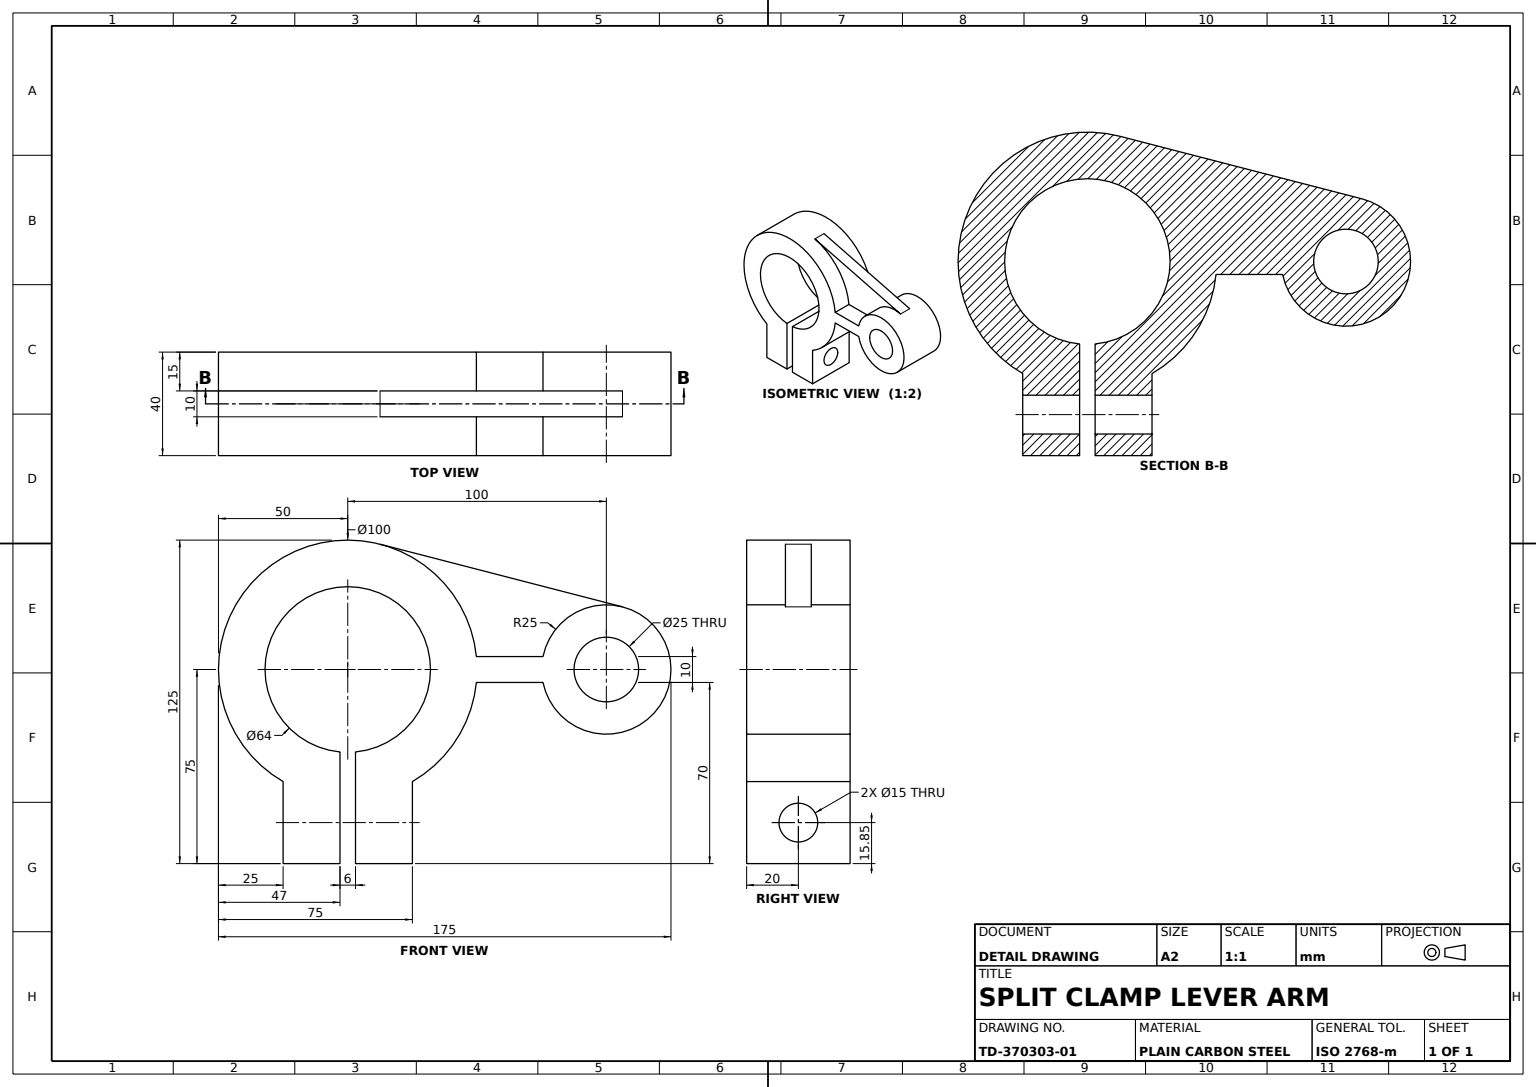
from build123d import *

# Parameters (mm, degrees)
CLAMP_RING_SKETCH_R                       = 50
CLAMP_RING_SKETCH_R_2                     = 32
CLAMP_RING_100_BORE_64_DEPTH              = 20
CLAMP_BLOCK_AND_SECONDARY_BOSS_SKETCH_R   = 25
CLAMP_BLOCK_AND_SECONDARY_BOSS_SKETCH_R_2 = 12.5
CLAMP_BLOCK_AND_SECONDARY_BOSS_SKETCH_W   = 50
CLAMP_BLOCK_AND_SECONDARY_BOSS_SKETCH_H   = 31.698729811
CLAMP_BLOCK_AND_SECONDARY_BOSS_DEPTH      = 20
CLAMP_SLOT_6MM_DEPTH                      = 148.139389696
CLAMP_SLOT_6MM_DEPTH_BACK                 = 148.139389696
CLAMP_SLOT_SKETCH_W                       = 6
CLAMP_SLOT_SKETCH_H                       = 43.140935356
CONNECTING_WEB_SKETCH_W                   = 55.5
CONNECTING_WEB_SKETCH_H                   = 10
CONNECTING_WEB_10MM_DEPTH                 = 20
STIFFENING_RIB_10MM_REACH                 = 149.139
STIFFENING_RIB_SKETCH_WALL_W              = 393.103363046
STIFFENING_RIB_SKETCH_WALL_H              = 10
CLAMP_BOLT_HOLE_15_DEPTH                  = 148.139389696
CLAMP_BOLT_HOLE_15_DEPTH_BACK             = 148.139389696
CLAMP_BOLT_HOLE_SKETCH_R                  = 7.5


with BuildPart() as part:
    # Clamp Ring Sketch → Clamp Ring Ø100 Bore Ø64 (new, symmetric)
    with BuildSketch(Plane.XY):
        Circle(CLAMP_RING_SKETCH_R)
        Circle(CLAMP_RING_SKETCH_R_2, mode=Mode.SUBTRACT)
    extrude(amount=CLAMP_RING_100_BORE_64_DEPTH, both=True)

    # Clamp Block and Secondary Boss Sketch → Clamp Block and Secondary Boss (add, symmetric)
    # profile 1 of 2: a face of its own
    with BuildSketch(Plane.XY):
        with Locations((100, 0)):
            Circle(CLAMP_BLOCK_AND_SECONDARY_BOSS_SKETCH_R)
        with Locations((100, 0)):
            Circle(CLAMP_BLOCK_AND_SECONDARY_BOSS_SKETCH_R_2, mode=Mode.SUBTRACT)
    # profile 2 of 2: a face of its own
    with BuildSketch(Plane.XY):
        with Locations((0, -59.150635095)):
            Rectangle(CLAMP_BLOCK_AND_SECONDARY_BOSS_SKETCH_W, CLAMP_BLOCK_AND_SECONDARY_BOSS_SKETCH_H)
    extrude(amount=CLAMP_BLOCK_AND_SECONDARY_BOSS_DEPTH, both=True)


with BuildPart() as clamp_block_and_secondary_boss_piece_1:
    # of the separate pieces the step leaves, piece 1, a body of its own (clamp_block_and_secondary_boss_pieces)
    add(part.part.solids().sort_by_distance((-25, -43.301270189, 20))[0])

    # Clamp Slot Sketch → Clamp Slot 6mm (cut, two sides: drawn at the far end of the back side and taken through both)
    with BuildSketch(Plane.XY.offset(-CLAMP_SLOT_6MM_DEPTH_BACK)):
        with Locations((0, -53.429532322)):
            Rectangle(CLAMP_SLOT_SKETCH_W, CLAMP_SLOT_SKETCH_H)
    extrude(amount=CLAMP_SLOT_6MM_DEPTH + CLAMP_SLOT_6MM_DEPTH_BACK, mode=Mode.SUBTRACT)



with BuildPart() as clamp_block_and_secondary_boss_piece_2:
    # of the separate pieces the step leaves, piece 2, a body of its own (clamp_block_and_secondary_boss_pieces)
    add(part.part.solids().sort_by_distance((125, 0, -20))[0])


with BuildPart() as clamp_block_and_secondary_boss_piece_1_1:
    add(clamp_block_and_secondary_boss_piece_1.part)

    add(clamp_block_and_secondary_boss_piece_2.part)  # Connecting Web 10mm merges Clamp Block and Secondary Boss piece 2
    # Connecting Web Sketch → Connecting Web 10mm (add, symmetric)
    with BuildSketch(Plane.XY):
        with Locations((59.75, 0)):
            Rectangle(CONNECTING_WEB_SKETCH_W, CONNECTING_WEB_SKETCH_H)
    extrude(amount=CONNECTING_WEB_10MM_DEPTH, both=True)

    # Stiffening Rib Sketch wall → Stiffening Rib 10mm (add, up to next)
    with BuildSketch(Plane(origin=(59.375, 36.309218871, 0), x_dir=(-0.968245836551, 0.250000000002, 0), z_dir=(-0.250000000002, -0.968245836551, 0)), mode=Mode.PRIVATE) as stiffening_rib_10mm_sk1:
        Rectangle(STIFFENING_RIB_SKETCH_WALL_W, STIFFENING_RIB_SKETCH_WALL_H)
    stiffening_rib_10mm_tool1 = extrude(stiffening_rib_10mm_sk1.sketch, amount=STIFFENING_RIB_10MM_REACH, mode=Mode.PRIVATE) - clamp_block_and_secondary_boss_piece_1_1.part
    add(stiffening_rib_10mm_tool1.solids().sort_by_distance((59.375, 36.309218871, 0))[0])

    # Clamp Bolt Hole Sketch → Clamp Bolt Hole Ø15 (cut, two sides: drawn at the far end of the back side and taken through both)
    with BuildSketch(Plane(origin=(0, 0, 0), x_dir=(0, 0, -1), z_dir=(1, 0, 0)).offset(-CLAMP_BOLT_HOLE_15_DEPTH_BACK)):
        with Locations(Location((0, -59.150635095, 0), (0, 0, 270))):
            Circle(CLAMP_BOLT_HOLE_SKETCH_R)
    extrude(amount=CLAMP_BOLT_HOLE_15_DEPTH + CLAMP_BOLT_HOLE_15_DEPTH_BACK, mode=Mode.SUBTRACT)


solid = clamp_block_and_secondary_boss_piece_1_1.part
